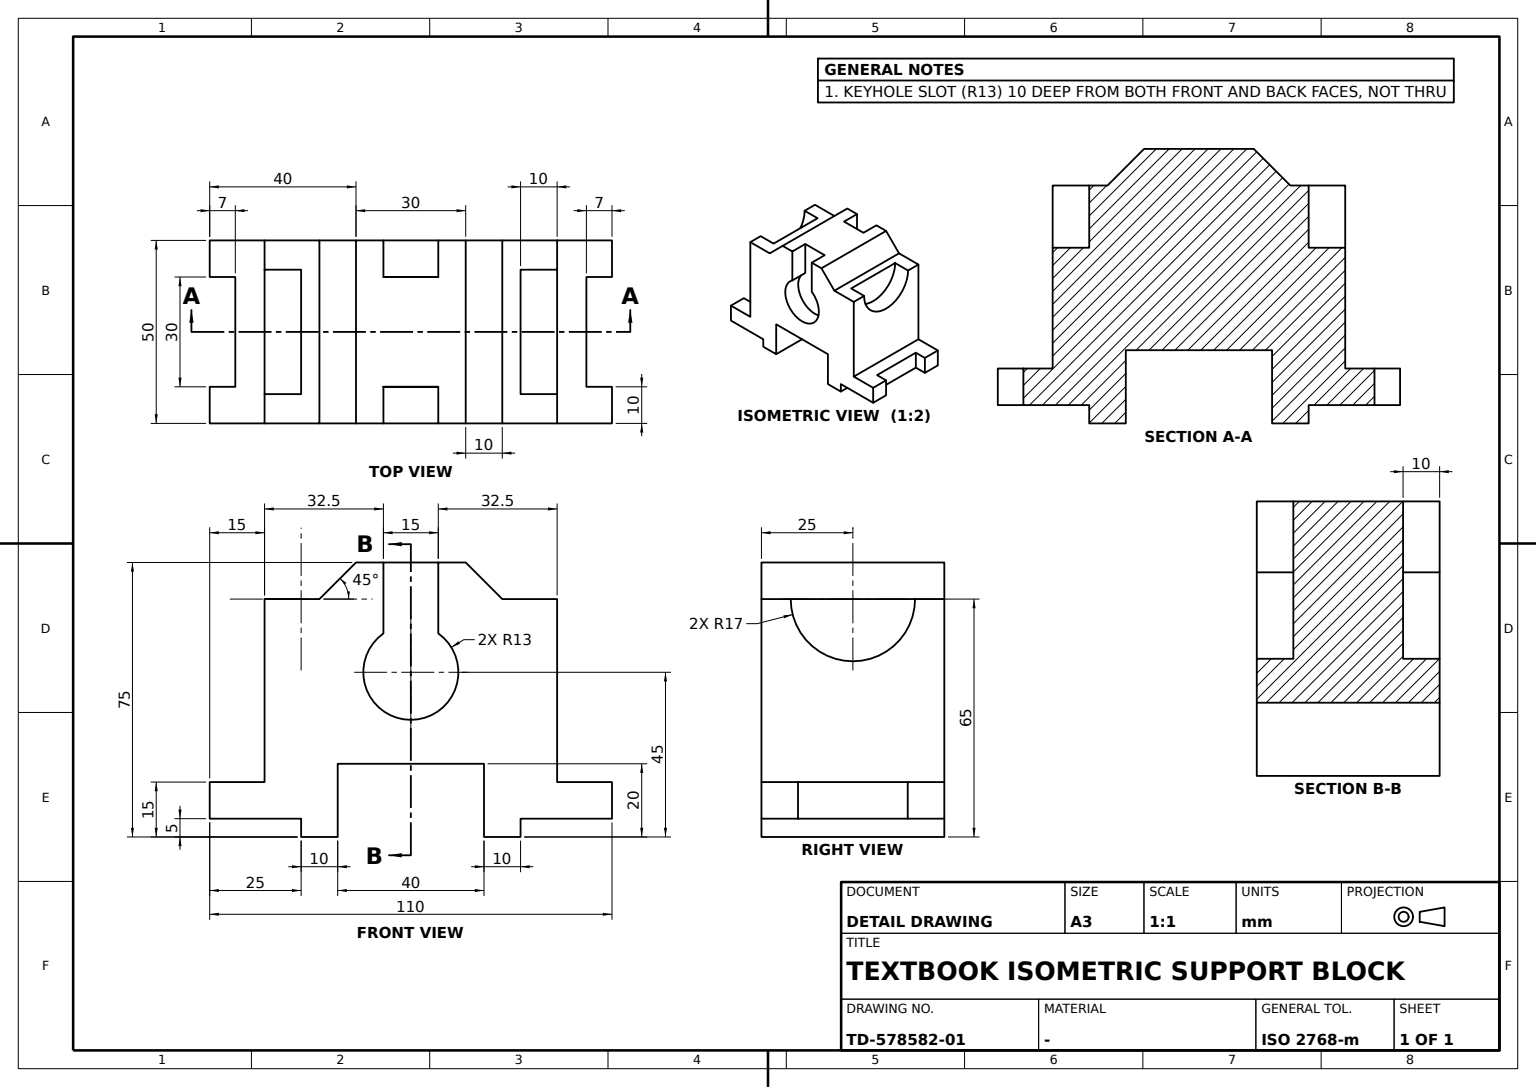
CATIA V5 part; units mm, degrees
sketch "Sketch1" plane through (0, 0, 0) normal (0, 1, 0) x (-1, 0, 0)
  line L0 (-25, 15) -> (-25, 5)
  line L1 (-25, 5) -> (0, 5)
  point P0 (0, 5)
  line L2 (0, 5) -> (0, 0)
  line L3 (0, 0) -> (10, 0)
  line L4 (10, 0) -> (10, 20)
  line L5 (10, 20) -> (50, 20)
  line L6 (50, 20) -> (50, 0)
  point P1 (50, 0)
  line L7 (50, 0) -> (60, 0)
  line L8 (60, 0) -> (60, 5)
  line L9 (60, 5) -> (85, 5)
  line L10 (85, 5) -> (85, 15)
  line L11 (85, 15) -> (70, 15)
  line L12 (70, 15) -> (70, 65)
  point P2 (70, 65)
  line L13 (-25, 15) -> (-10, 15)
  line L14 (-10, 15) -> (-10, 65)
  point P3 (-10, 65)
  line L15 (-10, 65) -> (5, 65)
  line L16 (30, 83.3753) -> (30, 0.5161) construction
  line L17 (70, 65) -> (55, 65)
  line L18 (15, 75) -> (45, 75)
  point P4 (30, 75)
  line L19 (5, 65) -> (15, 75)
  line L20 (55, 65) -> (45, 75)
  dimension "length L1" = 25
  dimension "length L0" = 10
  dimension "D3" = 5
  dimension "length L4" = 20
  dimension "length L8" = 5
  dimension "length L9" = 25
  dimension "length L10" = 10
  dimension "length L5" = 40
  dimension "length L11" = 15
  dimension "length L13" = 15
  dimension "distance L0 L10" = 110
  dimension "D12" = 10
  dimension "distance L7 P2" = 65
  dimension "distance L3 P3" = 65
  dimension "length L15" = 15
  dimension "length L18" = 30
  dimension "distance L18 L7" = 75
  constraint vertical L0 y-axis
  constraint vertical L2 y-axis
  constraint vertical L4 y-axis
  constraint vertical L6 y-axis
  constraint vertical L8 y-axis
  constraint vertical L10 y-axis
  constraint vertical L12 y-axis
  constraint vertical L14 y-axis
  constraint vertical L16 y-axis
  constraint coincidence P0 y-axis
  constraint coincidence P1 x-axis
  constraint coincidence P4 L16
  constraint horizontal L1 x-axis
  constraint horizontal L3 x-axis
  constraint horizontal L5 x-axis
  constraint horizontal L7 x-axis
  constraint horizontal L9 x-axis
  constraint horizontal L11 x-axis
  constraint horizontal L13 x-axis
  constraint horizontal L15 x-axis
  constraint horizontal L17 x-axis
  constraint horizontal L18 x-axis
  constraint symmetry L12 L14 L16
  constraint midpoint L18 P4
  constraint perpendicularity L20 L19
extrude "Pad1" add sketch "Sketch1" along normal mid plane 50
sketch "Sketch2" plane through (0, 25, 0) normal (0, 1, 0) x (-1, 0, 0)
  arc A0 (22.5, 55.6184) -> (37.5, 55.6184) centre (30, 45) ccw
  point P0 (30, 45)
  line L0 (22.5, 75) -> (37.5, 75)
  line L1 (37.5, 75) -> (37.5, 55.6184)
  line L2 (22.5, 55.6184) -> (22.5, 75)
  line L3 (45, 75) -> (15, 75) construction
  line L4 (50, 0) -> (60, 0) construction
  line L5 (70, 15) -> (70, 65) construction
  dimension "radius A0" = 13
  dimension "length L0" = 15
  dimension "distance P0 L4" = 45
  dimension "distance P0 L5" = 40
  constraint horizontal L0 x-axis
  constraint vertical L1 y-axis
  constraint vertical L2 y-axis
  constraint coincidence L0 L3
extrude "Pocket1" cut sketch "Sketch2" against normal blind 10
mirror "Mirror1" about plane through (0, 0, 0) normal (0, 1, 0) of "Pocket1"
sketch "Sketch3" plane through (10, 0, 0) normal (1, 0, 0) x (0, 1, 0)
  arc A0 (-17, 65) -> (17, 65) centre (0, 65) ccw
  point P0 (0, 65)
  line L0 (-25, 75) -> (25, 75) construction
  dimension "radius A0" = 17
  dimension "distance P0 L0" = 10
  constraint coincidence P0 y-axis
extrude "Pocket2" cut sketch "Sketch3" against normal blind 10 material side at (10, 0, 48.05)
sketch "Sketch4" plane through (-70, 0, 0) normal (-1, 0, 0) x (0, -1, 0)
  arc A0 (-17, 65) -> (17, 65) centre (0, 65) ccw
  point P0 (0, 65)
  line L0 (25, 75) -> (-25, 75) construction
  dimension "radius A0" = 17
  dimension "distance P0 L0" = 10
  constraint coincidence P0 y-axis
extrude "Pocket3" cut sketch "Sketch4" against normal blind 10 material side at (-70, 0, 48.05)
sketch "Sketch5" plane through (0, 0, 15) normal (0, 0, 1) x (0, 1, 0)
  line L0 (-15, 85) -> (15, 85)
  line L1 (15, 85) -> (15, 78)
  line L2 (15, 78) -> (-15, 78)
  line L3 (-15, 78) -> (-15, 85)
  line L4 (-25, 85) -> (25, 85) construction
  line L5 (25, 85) -> (25, 70) construction
  point P0 (0, 30.1136)
  line L6 (-15, -25) -> (15, -25)
  line L7 (15, -25) -> (15, -18)
  line L8 (15, -18) -> (-15, -18)
  line L9 (-15, -18) -> (-15, -25)
  line L10 (25, -10) -> (25, -25) construction
  line L11 (-25, -10) -> (-25, -25) construction
  line L12 (-25, -25) -> (25, -25) construction
  dimension "length L0" = 30
  dimension "length L1" = 7
  dimension "distance L1 L5" = 10
  dimension "distance L7 L10" = 10
  dimension "distance L9 L11" = 10
  dimension "length L8" = 30
  dimension "length L7" = 7
  constraint horizontal L0 x-axis
  constraint horizontal L2 x-axis
  constraint vertical L1 y-axis
  constraint vertical L3 y-axis
  constraint coincidence L0 L4
  constraint coincidence P0 y-axis
  constraint coincidence L6 L12
extrude "Pocket4" cut sketch "Sketch5" against normal blind 10
sketch "Sketch6" plane through (0, 25, 0) normal (0, 1, 0) x (-1, 0, 0)
properties part number "catia 24"
